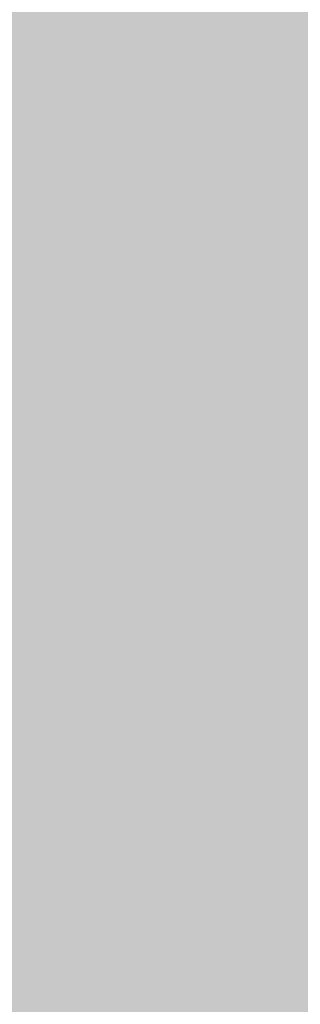
# Model space of a CAD drawing. Units: inches. Extents: x 2083 to 3317, y 1141 to 2115.
# Tile 167 of 256: x 3126.955939 to 3126.958245, y 1263.265937 to 1263.274018. Entities that reach past the tile are written whole.
import ezdxf

# ---------------------------------------------------------------- set-up
doc = ezdxf.new("R2010")
doc.units = ezdxf.units.IN
doc.layers.add('A-ANNO-DIMS', color=2, linetype='Continuous', lineweight=18)
doc.layers.add('A-WALL-PATT', color=251, linetype='Continuous', lineweight=13, true_color=0x636466)
doc.styles.get("Standard").update_dxf_attribs({"font": 'arial.ttf'})
doc.dimstyles.new('ISO-25', dxfattribs={"dimtxt": 12, "dimasz": 12, "dimexe": 1.25, "dimexo": 0.625, "dimtad": 1, "dimlunit": 3, "dimtxsty": 'Standard', "dimcen": 2.5, "dimadec": 0, "dimazin": 0, "dimtfac": 1, "dimtmove": 0, "dimatfit": 3, "dimfxl": 1, "dimarcsym": 0})

# ---------------------------------------------------------------- blocks, each defined once
blk = doc.blocks.new('*D26')
at = {"layer": 'A-ANNO-DIMS', "color": 0, "lineweight": -2, "transparency": 16777216}
for p, q in [((3088.985844, 1274.915092), (3088.985844, 1270.9519631)), ((3111.2400366, 1274.915092), (3111.2400366, 1270.9519631)), ((3076.985844, 1272.2019631), (2840.262447, 1272.2019631)), ((3111.2400366, 1272.2019631), (3088.985844, 1272.2019631)), ((3123.2400366, 1272.2019631), (3135.2400366, 1272.2019631))]:
    blk.add_line(p, q, dxfattribs=at)
at = {"layer": 'A-ANNO-DIMS', "color": 0, "transparency": 16777216}
for points in [[(3076.985844, 1274.2019631), (3076.985844, 1270.2019631), (3088.985844, 1272.2019631)], [(3123.2400366, 1274.2019631), (3123.2400366, 1270.2019631), (3111.2400366, 1272.2019631)]]:
    blk.add_solid(points, dxfattribs=at)
at = {"layer": 'Defpoints', "color": 0, "transparency": 16777216}
for p in [(3088.985844, 1275.540092), (3111.2400366, 1275.540092), (3088.985844, 1272.2019631)]:
    blk.add_point(p, dxfattribs=at)
at = {"layer": 'A-ANNO-DIMS', "color": 0, "transparency": 16777216, "insert": (2952.6241455, 1279.0316016), "char_height": 12, "attachment_point": 5}
blk.add_mtext('NIGHTSTAND 1\'-10 1/2" TYP.', dxfattribs=at)

msp = doc.modelspace()

# ---------------------------------------------------------------- hatches: boundary and pattern name
at = {"layer": 'A-WALL-PATT'}
h = msp.add_hatch(color=256, dxfattribs=at)
h.dxf.hatch_style = 1
h.paths.add_polyline_path([(3126.9597832, 2020.7613601), (2748.9597832, 2020.7613601), (2604.9597832, 2020.7613601), (2226.9597832, 2020.7613601), (2226.9597832, 1702.7613601), (2466.9597832, 1702.7613601), (2466.9597832, 1582.7613601), (2418.9597832, 1582.7613601), (2418.9597832, 1477.7613601), (2226.9597832, 1477.7613601), (2226.9597832, 1263.2613601), (2544.9597832, 1263.2613601), (2544.9597832, 1411.7613601), (2604.9597832, 1411.7613601), (2685.9597832, 1411.7613601), (2685.9597832, 1420.7613601), (2604.9597832, 1420.7613601), (2604.9597832, 1573.7613601), (2604.9597832, 1702.7613601), (2604.9597832, 2011.7613601), (2748.9597832, 2011.7613601), (2748.9597832, 1702.7613601), (2862.9597832, 1702.7613601), (2862.9597832, 1621.7613601), (2871.9597832, 1621.7613601), (2871.9597832, 1702.7613601), (2883.9597832, 1702.7613601), (2883.9597832, 1706.9394595, -0.026459), (2883.9597832, 1711.7613601), (2757.9597832, 1711.7613601), (2757.9597832, 1807.7613601), (2787.9597832, 1807.7613601), (2787.9597832, 1812.2613601), (2757.9597832, 1812.2613601), (2757.9597832, 2011.7613601), (2877.9597832, 2011.7613601), (2877.9597832, 1812.2613601), (2847.9597832, 1812.2613601), (2847.9597832, 1807.7613601), (2889.8357425, 1807.7613601), (2889.8357425, 1812.2613601), (2882.4597832, 1812.2613601), (2882.4597832, 2011.7613601), (3117.9597832, 2011.7613601), (3117.9597832, 1812.2613601), (2937.8357425, 1812.2613601), (2937.8357425, 1807.7613601), (2995.7097832, 1807.7613601), (2995.7097832, 1796.1176655), (3000.2097832, 1796.1176655), (3000.2097832, 1807.7613601), (3117.9597832, 1807.7613601), (3117.9597832, 1711.7613601), (3000.2097832, 1711.7613601), (3000.2097832, 1760.1176655), (2998.5727047, 1760.1176655, -0.020711), (2995.7097832, 1760.1176655), (2995.7097832, 1711.7613601), (2931.9597832, 1711.7613601), (2931.9597832, 1702.7613601), (3126.9597832, 1702.7613601)])
h.paths.add_polyline_path([(2471.4597832, 2011.7613601), (2471.4597832, 1810.0113601), (2462.7169357, 1810.0113601), (2462.7169357, 1805.5113601), (2505.9597832, 1805.5113601), (2505.9597832, 1810.0113601), (2475.9597832, 1810.0113601), (2475.9597832, 2011.7613601), (2595.9597832, 2011.7613601), (2595.9597832, 1810.0113601), (2565.9597832, 1810.0113601), (2565.9597832, 1805.5113601), (2595.9597832, 1805.5113601), (2595.9597832, 1711.7613601), (2235.9597832, 1711.7613601), (2235.9597832, 1805.5113601), (2353.7097832, 1805.5113601), (2353.7097832, 1796.0541624), (2358.2097832, 1796.0541624), (2358.2097832, 1805.5113601), (2414.7169357, 1805.5113601), (2414.7169357, 1810.0113601), (2235.9597832, 1810.0113601), (2235.9597832, 2011.7613601)], flags=16)
h.paths.add_polyline_path([(2270.2047343, 1994.6100082), (2270.2047343, 1970.6100082), (2246.2047343, 1970.6100082), (2246.2047343, 1994.6100082)], flags=0)
edge = h.paths.add_edge_path(flags=0)
edge.add_ellipse((2332.027391, 1899.7981761), major_axis=(-3.0429938, 3.0429938), ratio=0.16825245, start_angle=-161.3321656, end_angle=-156.3071136, ccw=False)
edge.add_ellipse((2333.0820373, 1898.7435297), major_axis=(-1.0546463, 1.0546463), ratio=0.453532097, start_angle=-123.371019, end_angle=-94.1591066)
edge = h.paths.add_edge_path(flags=0)
edge.add_ellipse((2332.027391, 1968.8762897), major_axis=(3.0429938, 3.0429938), ratio=0.16825245, start_angle=18.6678344, end_angle=23.6928864)
edge.add_spline(control_points=[(2332.9255964, 1970.6911045), (2332.2267681, 1970.3360997), (2330.8937087, 1969.6589054), (2328.4130803, 1970.9321376), (2327.2039345, 1967.7487119), (2324.7095965, 1969.9555886), (2322.5328223, 1967.012354), (2320.0128462, 1971.2958124), (2317.6803077, 1968.1578449), (2316.0405263, 1967.1020468), (2315.4269045, 1966.8096022)], knot_values=[0, 0, 0, 0, 2.267059, 4.324559, 6.685584, 8.878641, 11.121502, 14.300359, 17.755284, 19.732645, 19.732645, 19.732645, 19.732645], degree=3, periodic=0)
edge.add_ellipse((2332.027391, 1968.8762897), major_axis=(3.0429938, 3.0429938), ratio=0.16825245, start_angle=18.6678344, end_angle=23.6928864, ccw=False)
edge.add_ellipse((2333.0820373, 1969.930936), major_axis=(1.0546463, 1.0546463), ratio=0.453532097, start_angle=56.628981, end_angle=85.8408934, ccw=False)
edge = h.paths.add_edge_path(flags=0)
edge.add_spline(control_points=[(2296.4282874, 1967.9879081), (2293.6278045, 1965.3363137), (2287.7036238, 1959.727094), (2299.7438601, 1949.9956993), (2294.5325909, 1935.6685275), (2290.5732281, 1920.6035119), (2293.3941244, 1909.9736911), (2296.1854073, 1904.9665431)], knot_values=[0.099185, 0.099185, 0.099185, 0.099185, 0.345301, 0.619822, 0.982653, 1.386093, 1.810555, 1.810555, 1.810555, 1.810555], degree=3, periodic=0)
edge.add_spline(control_points=[(2296.1854073, 1904.9665431), (2297.3835817, 1902.6193002), (2298.0009694, 1901.9493116), (2298.5529698, 1901.4681549)], knot_values=[0.006246, 0.006246, 0.006246, 0.006246, 0.055476, 0.055476, 0.055476, 0.055476], degree=3, periodic=0)
edge.add_spline(control_points=[(2298.5529698, 1901.4681549), (2297.2586121, 1900.9232238), (2295.2252939, 1900.2321257), (2293.0602287, 1900.6142053), (2292.1014227, 1900.788415), (2292.0895776, 1900.790568)], knot_values=[0.312835, 0.312835, 0.312835, 0.312835, 0.40178, 0.474987, 0.475903, 0.475903, 0.475903, 0.475903], degree=3, periodic=0)
edge.add_arc((2292.7936464, 1904.6641088), 3.9370079, 215.4208969, 259.6981795, ccw=False)
edge.add_spline(control_points=[(2289.5853139, 1902.3823039), (2289.4766524, 1902.5350874), (2289.3684805, 1902.6880353), (2289.2608648, 1902.8411699)], knot_values=[0.102872, 0.102872, 0.102872, 0.102872, 0.116896, 0.116896, 0.116896, 0.116896], degree=3, periodic=0)
edge.add_spline(control_points=[(2289.2608648, 1902.8411699), (2288.6866042, 1902.5501922), (2287.6400477, 1902.0199025), (2285.8813368, 1901.8739536), (2283.8529717, 1901.5043521), (2281.7199871, 1899.7105375), (2278.4669913, 1899.492942), (2276.1571361, 1901.8832022), (2272.2589526, 1899.8040711), (2267.7776054, 1901.8431828), (2262.2438819, 1900.1840326), (2257.414927, 1901.7820606), (2254.318374, 1900.7261196), (2253.1782849, 1900.3373431)], knot_values=[0, 0, 0, 0, 1.907977, 3.477176, 5.261074, 7.972851, 11.680248, 13.717921, 16.939592, 22.789562, 27.502503, 33.595215, 37.145618, 37.145618, 37.145618, 37.145618], degree=3, periodic=0)
edge.add_line((2253.1782849, 1900.3373431), (2250.2442397, 1902.8411699))
edge.add_line((2250.2442397, 1902.8411699), (2250.2442397, 1965.8332959))
edge.add_line((2250.2442397, 1965.8332959), (2253.1782849, 1968.3371226))
edge.add_spline(control_points=[(2253.1782849, 1968.3371226), (2254.318374, 1967.9483462), (2257.414927, 1966.8924051), (2262.2438819, 1968.4904332), (2267.7776054, 1966.8312829), (2271.5267301, 1968.5372172), (2273.8759143, 1967.8282895), (2274.2067012, 1967.7276424)], knot_values=[0, 0, 0, 0, 0.09018, 0.244935, 0.364644, 0.513233, 0.537855, 0.537855, 0.537855, 0.537855], degree=3, periodic=0)
edge.add_arc((2274.3528869, 1963.7933495), 3.9370079, 72.0511336, 92.1279492, ccw=False)
edge.add_arc((2281.2969331, 1985.2300027), 18.5962982, 252.05113361, 288.56572166)
edge.add_arc((2292.3167172, 1956.0288805), 12.6460805, 71.02678788, 113.77821843, ccw=False)
edge = h.paths.add_edge_path(flags=0)
edge.add_spline(control_points=[(2274.8994147, 1951.8561946), (2275.066156, 1951.6165924), (2275.2326866, 1951.3765878), (2275.3979871, 1951.1358545)], knot_values=[1.409916, 1.409916, 1.409916, 1.409916, 1.43159, 1.43159, 1.43159, 1.43159], degree=3, periodic=0)
edge.add_spline(control_points=[(2275.3979871, 1951.1358545), (2275.7921055, 1950.5618854), (2276.1792311, 1949.9837745), (2276.5455462, 1949.3971029)], knot_values=[1.358238, 1.358238, 1.358238, 1.358238, 1.409916, 1.409916, 1.409916, 1.409916], degree=3, periodic=0)
edge.add_line((2276.5455462, 1949.3971029), (2277.437289, 1947.8621847))
edge.add_spline(control_points=[(2277.437289, 1947.8621847), (2276.3038341, 1945.6731147), (2274.6396979, 1942.4268817), (2274.631615, 1938.0938998), (2272.7991237, 1930.8515498), (2274.3564261, 1943.8970461), (2275.9476814, 1947.9233558), (2276.5455462, 1949.3971029)], knot_values=[0.005632, 0.005632, 0.005632, 0.005632, 0.186014, 0.266002, 0.357087, 0.59639, 0.739732, 0.739732, 0.739732, 0.739732], degree=3, periodic=0)
edge.add_spline(control_points=[(2276.5455462, 1949.3971029), (2276.1792311, 1949.9837745), (2275.7921055, 1950.5618854), (2275.3979871, 1951.1358545)], knot_values=[1.358238, 1.358238, 1.358238, 1.358238, 1.409916, 1.409916, 1.409916, 1.409916], degree=3, periodic=0)
edge.add_spline(control_points=[(2275.3979871, 1951.1358545), (2274.9425002, 1950.0804523), (2274.2077604, 1948.0252718), (2273.9346018, 1944.8514774), (2272.4685341, 1937.6274891), (2273.4662155, 1945.6964663), (2274.7006154, 1951.0594725), (2274.8994147, 1951.8561946)], knot_values=[0.104364, 0.104364, 0.104364, 0.104364, 0.189636, 0.269624, 0.36071, 0.600013, 0.644622, 0.644622, 0.644622, 0.644622], degree=3, periodic=0)
h.paths.add_polyline_path([(2269.1675139, 1963.1275729, -0.357527), (2268.170633, 1960.9763695, -0.092561), (2268.170633, 1939.4363249, -0.357527), (2269.1675139, 1937.2851215, -0.357527), (2267.0163105, 1938.2820024, -0.164785), (2254.6855813, 1938.2820024, -0.357527), (2252.5343779, 1937.2851215, -0.357527), (2253.5312587, 1939.4363249, -0.092561), (2253.5312587, 1960.9763695, -0.357527), (2252.5343779, 1963.1275729, -0.357527), (2254.6855813, 1962.130692, -0.164785), (2267.0163105, 1962.130692, -0.357527)], flags=0)
h.paths.add_polyline_path([(2248.8740679, 1967.8017998), (2248.8740679, 1957.0277095), (2249.4577833, 1957.0277095), (2249.4577833, 1911.6467562), (2248.8740679, 1911.6467562), (2248.8740679, 1900.8726659), (2246.5118632, 1900.8726659, 0.197327), (2244.1496584, 1902.4568734), (2244.1496584, 1966.2175923, 0.197327), (2246.5118632, 1967.8017998)], flags=0)
h.paths.add_polyline_path([(2269.1675139, 1931.3893442, -0.357527), (2268.170633, 1929.2381408, -0.092561), (2268.170633, 1907.6980962, -0.357527), (2269.1675139, 1905.5468928, -0.357527), (2267.0163105, 1906.5437737, -0.164785), (2254.6855813, 1906.5437737, -0.357527), (2252.5343779, 1905.5468928, -0.357527), (2253.5312587, 1907.6980962, -0.092561), (2253.5312587, 1929.2381408, -0.357527), (2252.5343779, 1931.3893442, -0.357527), (2254.6855813, 1930.3924634, -0.164785), (2267.0163105, 1930.3924634, -0.357527)], flags=0)
edge = h.paths.add_edge_path(flags=0)
edge.add_spline(control_points=[(2276.1968578, 1906.7237016), (2276.1681442, 1909.0289278), (2276.1140492, 1913.371852), (2270.5984171, 1924.9249783), (2273.9051746, 1919.0127787), (2275.9217115, 1916.2620626), (2275.4745699, 1912.4021495), (2277.2578735, 1910.3806206), (2276.6960436, 1908.2250358), (2276.6462176, 1906.8130226), (2276.6178249, 1906.0084068)], knot_values=[0, 0, 0, 0, 8.61026, 16.221274, 18.843057, 23.804898, 27.440828, 29.356102, 31.203478, 33.650687, 33.650687, 33.650687, 33.650687], degree=3, periodic=0)
edge.add_spline(control_points=[(2276.6178249, 1906.0084068), (2276.6233131, 1905.6241436), (2276.4977381, 1904.6286608), (2275.4417789, 1903.8547251), (2274.9373144, 1903.0804497), (2274.8590804, 1902.8411699)], knot_values=[0.156488, 0.156488, 0.156488, 0.156488, 0.184398, 0.231376, 0.250598, 0.250598, 0.250598, 0.250598], degree=3, periodic=0)
edge.add_line((2274.8590804, 1902.8411699), (2276.50598, 1902.8411699))
edge.add_spline(control_points=[(2276.50598, 1902.8411699), (2276.7883084, 1903.0849395), (2277.6650711, 1904.1251958), (2278.2495378, 1904.340738), (2277.6538719, 1908.5273866), (2278.15567, 1906.2278078), (2278.100464, 1905.2859484), (2278.8466748, 1904.0690054), (2277.8567853, 1903.4149482), (2277.8741909, 1902.9910497), (2277.9035616, 1902.8411699)], knot_values=[0.059574, 0.059574, 0.059574, 0.059574, 0.080753, 0.103741, 0.16972, 0.176036, 0.207137, 0.240474, 0.262341, 0.27366, 0.27366, 0.27366, 0.27366], degree=3, periodic=0)
edge.add_line((2277.9035616, 1902.8411699), (2280.0298255, 1902.8411699))
edge.add_spline(control_points=[(2280.0298255, 1902.8411699), (2279.8882214, 1903.088398), (2279.4992571, 1903.9815512), (2280.1522839, 1905.9393491), (2278.103615, 1909.6577572), (2279.7623946, 1907.185285), (2280.3279002, 1904.8748608), (2280.4851086, 1903.4895904), (2281.4632687, 1903.2494323), (2281.7583431, 1902.9364967), (2281.8340361, 1902.8411699)], knot_values=[0.013856, 0.013856, 0.013856, 0.013856, 0.034874, 0.088867, 0.107879, 0.126738, 0.158714, 0.193757, 0.217487, 0.226722, 0.226722, 0.226722, 0.226722], degree=3, periodic=0)
edge.add_spline(control_points=[(2281.8340361, 1902.8411699), (2281.7875348, 1902.8267029), (2281.6470224, 1902.7829881), (2281.3955272, 1902.85949), (2281.088077, 1902.9852418), (2280.7206826, 1903.060902), (2280.3334513, 1903.0257257), (2280.1247668, 1902.898879), (2280.0298255, 1902.8411699)], knot_values=[0, 0, 0, 0, 0.14413, 0.435517, 0.749276, 1.153046, 1.548371, 1.878348, 1.878348, 1.878348, 1.878348], degree=3, periodic=0)
edge.add_line((2280.0298255, 1902.8411699), (2277.9035616, 1902.8411699))
edge.add_spline(control_points=[(2277.9035616, 1902.8411699), (2277.892855, 1902.7958553), (2277.865396, 1902.6796374), (2277.6074793, 1902.6874828), (2277.2740503, 1902.8006999), (2276.8379209, 1902.6197745), (2276.5838074, 1902.7892611), (2276.50598, 1902.8411699)], knot_values=[0, 0, 0, 0, 0.127189, 0.326199, 0.628009, 1.24357, 1.515331, 1.515331, 1.515331, 1.515331], degree=3, periodic=0)
edge.add_line((2276.50598, 1902.8411699), (2274.8590804, 1902.8411699))
edge.add_spline(control_points=[(2274.8590804, 1902.8411699), (2274.8144367, 1902.8985868), (2274.7251297, 1903.013446), (2274.4934765, 1903.1189684), (2274.2442854, 1902.9605386), (2273.9371207, 1903.1849416), (2273.6140395, 1902.9831428), (2273.4083164, 1902.8830449), (2273.322254, 1902.8411699)], knot_values=[0, 0, 0, 0, 0.21843, 0.436957, 0.687977, 0.990379, 1.398396, 1.69185, 1.69185, 1.69185, 1.69185], degree=3, periodic=0)
edge.add_spline(control_points=[(2273.322254, 1902.8411699), (2273.6167403, 1903.445692), (2274.2739977, 1904.5382529), (2276.0272387, 1904.5737017), (2276.2069634, 1906.5836372), (2276.1968578, 1906.7237016)], knot_values=[0.012227, 0.012227, 0.012227, 0.012227, 0.059472, 0.106218, 0.134458, 0.134458, 0.134458, 0.134458], degree=3, periodic=0)
h.paths.add_polyline_path([(2270.7760538, 1897.7898284), (2270.7760538, 1873.7898284), (2246.7760538, 1873.7898284), (2246.7760538, 1897.7898284)], flags=0)
h.paths.add_polyline_path([(2353.7097832, 1760.0050593), (2353.7097832, 1760.0541624), (2358.2097832, 1760.0541624, -0.033729)], flags=0)
h.paths.add_polyline_path([(2321.8191188, 1737.5291862), (2341.9953271, 1737.5291862, -0.414214), (2343.2032727, 1736.3212406), (2343.2032727, 1721.0205964, -0.414214), (2341.9953271, 1719.8126508), (2321.8191188, 1719.8126508, -0.414214), (2320.6111732, 1721.0205964), (2320.6111732, 1736.3212406, -0.414214)], flags=0)
h.paths.add_polyline_path([(2324.2350099, 1736.3212406), (2339.5794359, 1736.3212406, -0.414214), (2341.9953271, 1733.9053494), (2341.9953271, 1725.4497302, -0.414214), (2339.5794359, 1723.033839), (2333.6805885, 1723.033839), (2333.8453172, 1722.0454666, -0.870646), (2335.4253988, 1721.8258934, -0.767327), (2333.922694, 1721.4232449), (2331.2910241, 1721.4232449, -0.767327), (2329.7883193, 1721.8258934, -0.870646), (2331.3684009, 1722.0454666), (2331.5331296, 1723.033839), (2324.2350099, 1723.033839, -0.414214), (2321.8191188, 1725.4497302), (2321.8191188, 1733.9053494, -0.414214)], flags=0)
h.paths.add_polyline_path([(2570.4837892, 1928.6154443), (2589.6837892, 1928.6154443), (2590.1688286, 1928.6154443), (2590.1688286, 1904.9933971), (2570.4837892, 1904.9933971)], flags=0)
h.paths.add_polyline_path([(2574.4473242, 1927.2638215, -1), (2572.8288357, 1927.2638215, -1)], flags=0)
h.paths.add_polyline_path([(2573.0898665, 1926.9408768), (2573.925032, 1927.7760423), (2574.1477428, 1927.5533315), (2573.3125773, 1926.718166)], flags=0)
h.paths.add_polyline_path([(2578.7790648, 1919.7296175, -1), (2571.5916632, 1919.7296175, -1)], flags=0)
h.paths.add_polyline_path([(2578.385364, 1919.7296175, -1), (2571.985364, 1919.7296175, -1)], flags=0)
h.paths.add_polyline_path([(2331.5957638, 1729.4762156, -1), (2333.6179542, 1729.4762156, -1)], flags=0)
h.paths.add_polyline_path([(2578.0342282, 1927.2638215, -1), (2576.4157396, 1927.2638215, -1)], flags=0)
h.paths.add_polyline_path([(2576.6888513, 1927.5310886), (2576.9115621, 1927.7537993), (2577.7467276, 1926.9186339), (2577.5240168, 1926.6959231)], flags=0)
h.paths.add_polyline_path([(2578.1390648, 1909.8595388, -1), (2572.2316632, 1909.8595388, -1)], flags=0)
h.paths.add_polyline_path([(2577.745364, 1909.8595388, -1), (2572.625364, 1909.8595388, -1)], flags=0)
h.paths.add_polyline_path([(2583.7977179, 1927.2638215, -1), (2582.1792294, 1927.2638215, -1)], flags=0)
h.paths.add_polyline_path([(2582.7186487, 1927.7537993), (2583.5538142, 1926.9186339), (2583.3311034, 1926.6959231), (2582.4959379, 1927.5310886)], flags=0)
h.paths.add_polyline_path([(2582.4959379, 1927.5310886), (2582.7186487, 1927.7537993), (2583.5538142, 1926.9186339), (2583.3311034, 1926.6959231)], flags=0)
h.paths.add_polyline_path([(2587.7390648, 1920.5296175, -1), (2581.8316632, 1920.5296175, -1)], flags=0)
h.paths.add_polyline_path([(2587.345364, 1920.5296175, -1), (2582.225364, 1920.5296175, -1)], flags=0)
h.paths.add_polyline_path([(2587.3846219, 1927.2638215, -1), (2585.7661333, 1927.2638215, -1)], flags=0)
h.paths.add_polyline_path([(2586.0819925, 1926.9802469), (2586.917158, 1927.8154124), (2587.1398688, 1927.5927016), (2586.3047033, 1926.7575361)], flags=0)
h.paths.add_polyline_path([(2588.3790648, 1910.6595388, -1), (2581.1916632, 1910.6595388, -1)], flags=0)
h.paths.add_polyline_path([(2587.985364, 1910.6595388, -1), (2581.585364, 1910.6595388, -1)], flags=0)
h.paths.add_polyline_path([(2417.1677288, 1729.4778955), (2437.3439372, 1729.4778955, -0.414214), (2438.5518828, 1728.2699499), (2438.5518828, 1712.9693057, -0.414214), (2437.3439372, 1711.7613601), (2417.1677288, 1711.7613601, -0.414214), (2415.9597832, 1712.9693057), (2415.9597832, 1728.2699499, -0.414214)], flags=0)
h.paths.add_polyline_path([(2419.58362, 1728.2699499), (2434.928046, 1728.2699499, -0.414214), (2437.3439372, 1725.8540587), (2437.3439372, 1717.3984395, -0.414214), (2434.928046, 1714.9825483), (2429.0291985, 1714.9825483), (2429.1939273, 1713.9941758, -0.870646), (2430.7740089, 1713.7746027, -0.767327), (2429.2713041, 1713.3719542), (2426.6396342, 1713.3719542, -0.767327), (2425.1369294, 1713.7746027, -0.870646), (2426.717011, 1713.9941758), (2426.8817397, 1714.9825483), (2419.58362, 1714.9825483, -0.414214), (2417.1677288, 1717.3984395), (2417.1677288, 1725.8540587, -0.414214)], flags=0)
h.paths.add_polyline_path([(2419.58362, 1728.2699499), (2434.928046, 1728.2699499, -0.414214), (2437.3439372, 1725.8540587), (2437.3439372, 1717.3984395, -0.414214), (2434.928046, 1714.9825483), (2429.0291985, 1714.9825483), (2428.3581177, 1719.0090337), (2427.5528206, 1719.0090337), (2426.8817397, 1714.9825483), (2419.58362, 1714.9825483, -0.414214), (2417.1677288, 1717.3984395), (2417.1677288, 1725.8540587, -0.414214)], flags=0)
h.paths.add_polyline_path([(2426.9443739, 1721.4249248, -1), (2428.9665643, 1721.4249248, -1)], flags=0)
h.paths.add_polyline_path([(2475.9597832, 1702.7613601), (2595.9597832, 1702.7613601), (2595.9597832, 1582.7613601), (2475.9597832, 1582.7613601)], flags=16)
h.paths.add_polyline_path([(2427.9597832, 1573.7613601), (2595.9597832, 1573.7613601), (2595.9597832, 1468.7613601), (2595.9597832, 1420.7613601), (2384.4597832, 1420.7613601), (2384.4597832, 1468.7613601), (2427.9597832, 1468.7613601)], flags=16)
h.paths.add_polyline_path([(2379.9597832, 1468.7613601), (2379.9597832, 1420.7613601), (2235.9597832, 1420.7613601), (2235.9597832, 1468.7613601)], flags=16)
h.paths.add_polyline_path([(2317.8159962, 1466.695767), (2337.9922045, 1466.695767, -0.414214), (2339.2001501, 1465.4878214), (2339.2001501, 1450.1871771, -0.414214), (2337.9922045, 1448.9792315), (2317.8159962, 1448.9792315, -0.414214), (2316.6080506, 1450.1871771), (2316.6080506, 1465.4878214, -0.414214)], flags=0)
h.paths.add_polyline_path([(2320.2318874, 1465.4878214), (2335.5763133, 1465.4878214, -0.414214), (2337.9922045, 1463.0719302), (2337.9922045, 1454.616311, -0.414214), (2335.5763133, 1452.2004198), (2329.6774659, 1452.2004198), (2329.8421946, 1451.2120473, -0.870646), (2331.4222762, 1450.9924742, -0.767327), (2329.9195714, 1450.5898257), (2327.2879015, 1450.5898257, -0.767327), (2325.7851967, 1450.9924742, -0.870646), (2327.3652783, 1451.2120473), (2327.530007, 1452.2004198), (2320.2318874, 1452.2004198, -0.414214), (2317.8159962, 1454.616311), (2317.8159962, 1463.0719302, -0.414214)], flags=0)
h.paths.add_polyline_path([(2320.2318874, 1465.4878214), (2335.5763133, 1465.4878214, -0.414214), (2337.9922045, 1463.0719302), (2337.9922045, 1454.616311, -0.414214), (2335.5763133, 1452.2004198), (2329.6774659, 1452.2004198), (2329.006385, 1456.2269051), (2328.2010879, 1456.2269051), (2327.530007, 1452.2004198), (2320.2318874, 1452.2004198, -0.414214), (2317.8159962, 1454.616311), (2317.8159962, 1463.0719302, -0.414214)], flags=0)
h.paths.add_polyline_path([(2327.5926413, 1458.6427963, -1), (2329.6148317, 1458.6427963, -1)], flags=0)
h.paths.add_polyline_path([(2244.4117436, 1433.3404531), (2241.9209449, 1433.3404531, -0.414214), (2240.0178562, 1435.2435418), (2240.0178562, 1440.9528078, -0.414211), (2241.920925, 1442.8558965), (2244.4117436, 1442.8558965, -1.976472)], flags=0)
h.paths.add_polyline_path([(2245.3568884, 1434.3975358, -0.414214), (2245.3568884, 1441.7988138, -2.144098)], flags=0)
h.paths.add_polyline_path([(2535.9597832, 1416.2613601), (2535.9597832, 1272.2613601), (2235.9597832, 1272.2613601), (2235.9597832, 1416.2613601)], flags=16)
h.paths.add_polyline_path([(2260.1195614, 1384.2928413), (2260.1195614, 1362.0386487), (2237.8653688, 1362.0386487), (2237.8653688, 1384.2928413)], flags=0)
edge = h.paths.add_edge_path(flags=0)
edge.add_line((2318.2518466, 1362.0932983), (2318.1457968, 1362.0009726))
edge.add_ellipse((2317.4451158, 1360.4310442), major_axis=(2.8216404, 2.8216404), ratio=0.16825245, start_angle=18.6678344, end_angle=20.9481273, ccw=False)
edge.add_ellipse((2318.4230451, 1361.4089735), major_axis=(0.9779293, 0.9779293), ratio=0.453532097, start_angle=56.628981, end_angle=70.2262012, ccw=False)
edge = h.paths.add_edge_path(flags=0)
edge.add_line((2319.1073699, 1295.5710784), (2319.0150442, 1295.6771282))
edge.add_ellipse((2317.4451158, 1296.3778091), major_axis=(-2.8216404, 2.8216404), ratio=0.16825245, start_angle=-161.3321656, end_angle=-159.0518727, ccw=False)
edge.add_ellipse((2318.4230451, 1295.3998798), major_axis=(-0.9779293, 0.9779293), ratio=0.453532097, start_angle=-123.371019, end_angle=-109.7737988)
edge = h.paths.add_edge_path(flags=0)
edge.add_spline(control_points=[(2284.2103489, 1301.1702189), (2284.5806878, 1300.444719), (2284.8911891, 1299.8920243), (2285.159553, 1299.4610182)], knot_values=[0.039066, 0.039066, 0.039066, 0.039066, 0.055476, 0.055476, 0.055476, 0.055476], degree=3, periodic=0)
edge.add_line((2285.159553, 1299.4610182), (2284.2103489, 1301.1702189))
edge = h.paths.add_edge_path(flags=0)
edge.add_line((2280.4124579, 1297.2980125), (2283.3699905, 1297.0361216))
edge.add_line((2283.3699905, 1297.0361216), (2286.4056902, 1297.9263104))
edge.add_spline(control_points=[(2286.4056902, 1297.9263104), (2285.305487, 1297.4631193), (2284.3447774, 1297.1291508), (2283.3699905, 1297.0361216)], knot_values=[0.394369, 0.394369, 0.394369, 0.394369, 0.475903, 0.475903, 0.475903, 0.475903], degree=3, periodic=0)
edge.add_spline(control_points=[(2283.3699905, 1297.0361216), (2283.2813895, 1297.027666), (2282.316289, 1296.9573356), (2281.3125019, 1297.1344787), (2280.4234414, 1297.2960161), (2280.4124579, 1297.2980125)], knot_values=[0.312835, 0.312835, 0.312835, 0.312835, 0.320246, 0.393453, 0.394369, 0.394369, 0.394369, 0.394369], degree=3, periodic=0)
edge = h.paths.add_edge_path(flags=0)
edge.add_line((2284.4355615, 1359.6072854), (2280.4462909, 1355.328047))
edge.add_line((2280.4462909, 1355.328047), (2279.5799868, 1351.0177544))
edge.add_line((2279.5799868, 1351.0177544), (2282.4129737, 1346.5804327))
edge.add_spline(control_points=[(2282.4129737, 1346.5804327), (2283.1533308, 1345.5892358), (2284.2528957, 1344.0288973), (2284.801037, 1342.3871671), (2284.9351625, 1341.8055443)], knot_values=[1.240098, 1.240098, 1.240098, 1.240098, 1.332892, 1.382712, 1.382712, 1.382712, 1.382712], degree=3, periodic=0)
edge.add_spline(control_points=[(2284.9351625, 1341.8055443), (2285.3191079, 1340.1406002), (2285.2330291, 1338.4092041), (2284.9099384, 1336.6541222)], knot_values=[1.097484, 1.097484, 1.097484, 1.097484, 1.240098, 1.240098, 1.240098, 1.240098], degree=3, periodic=0)
edge.add_spline(control_points=[(2284.9099384, 1336.6541222), (2284.5868478, 1334.8990403), (2284.0267453, 1333.1202725), (2283.4626437, 1331.3605849)], knot_values=[0.95487, 0.95487, 0.95487, 0.95487, 1.097484, 1.097484, 1.097484, 1.097484], degree=3, periodic=0)
edge.add_line((2283.4626437, 1331.3605849), (2281.8903759, 1326.153357))
edge.add_line((2281.8903759, 1326.153357), (2280.7562592, 1321.0560888))
edge.add_line((2280.7562592, 1321.0560888), (2280.2992048, 1316.0019772))
edge.add_line((2280.2992048, 1316.0019772), (2280.7159327, 1310.9500678))
edge.add_line((2280.7159327, 1310.9500678), (2282.0280939, 1305.9721367))
edge.add_line((2282.0280939, 1305.9721367), (2284.2103489, 1301.1702189))
edge.add_spline(control_points=[(2284.2103489, 1301.1702189), (2283.3407305, 1302.7301854), (2282.6119044, 1304.3364933), (2282.0280939, 1305.9721367)], knot_values=[0.099185, 0.099185, 0.099185, 0.099185, 0.241799, 0.241799, 0.241799, 0.241799], degree=3, periodic=0)
edge.add_spline(control_points=[(2282.0280939, 1305.9721367), (2281.4442835, 1307.6077801), (2281.0054886, 1309.2727591), (2280.7159327, 1310.9500678)], knot_values=[0.241799, 0.241799, 0.241799, 0.241799, 0.384413, 0.384413, 0.384413, 0.384413], degree=3, periodic=0)
edge.add_spline(control_points=[(2280.7159327, 1310.9500678), (2280.4332411, 1312.5876134), (2280.2893863, 1314.2769594), (2280.2988938, 1315.9620324), (2280.2992048, 1316.0019772)], knot_values=[0.384413, 0.384413, 0.384413, 0.384413, 0.523647, 0.527028, 0.527028, 0.527028, 0.527028], degree=3, periodic=0)
edge.add_spline(control_points=[(2280.2992048, 1316.0019772), (2280.3123257, 1317.6869552), (2280.4778706, 1319.3679256), (2280.7562592, 1321.0560888)], knot_values=[0.527028, 0.527028, 0.527028, 0.527028, 0.669642, 0.669642, 0.669642, 0.669642], degree=3, periodic=0)
edge.add_spline(control_points=[(2280.7562592, 1321.0560888), (2281.0346478, 1322.7442519), (2281.4258801, 1324.4396079), (2281.8903759, 1326.153357)], knot_values=[0.669642, 0.669642, 0.669642, 0.669642, 0.812256, 0.812256, 0.812256, 0.812256], degree=3, periodic=0)
edge.add_spline(control_points=[(2281.8903759, 1326.153357), (2282.2643834, 1327.5332507), (2282.7878702, 1329.2618097), (2283.352751, 1331.0177803), (2283.4626437, 1331.3605849)], knot_values=[0.812256, 0.812256, 0.812256, 0.812256, 0.927087, 0.95487, 0.95487, 0.95487, 0.95487], degree=3, periodic=0)
edge.add_line((2283.4626437, 1331.3605849), (2284.9099384, 1336.6541222))
edge.add_line((2284.9099384, 1336.6541222), (2284.9351625, 1341.8055443))
edge.add_line((2284.9351625, 1341.8055443), (2282.4129737, 1346.5804327))
edge.add_spline(control_points=[(2282.4129737, 1346.5804327), (2281.2751273, 1348.1037918), (2280.0784467, 1349.5703178), (2279.5799868, 1351.0177544)], knot_values=[1.382712, 1.382712, 1.382712, 1.382712, 1.525326, 1.525326, 1.525326, 1.525326], degree=3, periodic=0)
edge.add_spline(control_points=[(2279.5799868, 1351.0177544), (2279.4432818, 1351.4147209), (2279.1363124, 1352.856922), (2279.7351897, 1354.2903851), (2280.4462909, 1355.328047)], knot_values=[1.525326, 1.525326, 1.525326, 1.525326, 1.564439, 1.667941, 1.667941, 1.667941, 1.667941], degree=3, periodic=0)
edge.add_spline(control_points=[(2280.4462909, 1355.328047), (2281.4261132, 1356.7578354), (2282.9308373, 1358.1825604), (2284.4355615, 1359.6072854)], knot_values=[1.667941, 1.667941, 1.667941, 1.667941, 1.810555, 1.810555, 1.810555, 1.810555], degree=3, periodic=0)
edge.add_arc((2280.6230749, 1348.518181), 11.7261796, 71.02678788, 113.77821843)
edge.add_arc((2270.4048917, 1375.5951559), 17.2435667, 252.05113361, 288.56572166, ccw=False)
edge.add_arc((2263.9659692, 1355.7178471), 3.6506221, 72.0511336, 92.1279492)
edge.add_arc((2263.9659692, 1355.7178471), 3.6506221, 92.1279492, 177.98513)
edge.add_spline(control_points=[(2260.3176041, 1355.8461989), (2260.2604169, 1354.2206683), (2260.551278, 1350.1865469), (2262.9993445, 1346.7662507), (2264.4727415, 1344.6490245)], knot_values=[1.43159, 1.43159, 1.43159, 1.43159, 1.564144, 1.770695, 1.770695, 1.770695, 1.770695], degree=3, periodic=0)
edge.add_line((2264.4727415, 1344.6490245), (2264.9355904, 1343.9825301))
edge.add_spline(control_points=[(2263.8010444, 1340.2481052), (2263.8432379, 1340.5140884), (2264.0672444, 1341.7564652), (2264.5126928, 1343.0024532), (2264.9350468, 1343.9810834)], knot_values=[0.53657, 0.53657, 0.53657, 0.53657, 0.559349, 0.644622, 0.644622, 0.644622, 0.644622], degree=3, periodic=0)
edge.add_spline(control_points=[(2264.9350468, 1343.9810834), (2265.1177715, 1343.7149747), (2265.2988751, 1343.4479058), (2265.4767562, 1343.1793646)], knot_values=[1.384077, 1.384077, 1.384077, 1.384077, 1.409916, 1.409916, 1.409916, 1.409916], degree=3, periodic=0)
edge.add_spline(control_points=[(2265.4767562, 1343.1793646), (2265.6546373, 1342.9108234), (2265.8292958, 1342.64081), (2265.9991301, 1342.368812)], knot_values=[1.358238, 1.358238, 1.358238, 1.358238, 1.384077, 1.384077, 1.384077, 1.384077], degree=3, periodic=0)
edge.add_line((2265.9991301, 1342.368812), (2266.8260057, 1340.9455468))
edge.add_spline(control_points=[(2266.8260057, 1340.9455468), (2268.894401, 1337.0896912), (2271.3981727, 1325.8430009), (2270.5161644, 1310.5685568), (2275.9193759, 1301.860609), (2277.7895113, 1299.1994495)], knot_values=[0.116896, 0.116896, 0.116896, 0.116896, 0.472987, 1.050969, 1.313793, 1.313793, 1.313793, 1.313793], degree=3, periodic=0)
edge.add_spline(control_points=[(2277.7895113, 1299.1994495), (2277.8394051, 1299.1284519), (2277.8894277, 1299.0574975), (2277.9395717, 1298.9865839)], knot_values=[0.109884, 0.109884, 0.109884, 0.109884, 0.116896, 0.116896, 0.116896, 0.116896], degree=3, periodic=0)
edge.add_line((2277.9395717, 1298.9865839), (2277.7888489, 1299.1991139))
edge.add_spline(control_points=[(2277.7888489, 1299.1991139), (2277.2565819, 1298.9294144), (2276.2863504, 1298.4379024), (2275.0393517, 1298.3344186), (2274.3833299, 1298.2388951), (2274.2152543, 1298.209338)], knot_values=[33.12187, 33.12187, 33.12187, 33.12187, 35.029056, 36.598255, 37.144827, 37.144827, 37.144827, 37.144827], degree=3, periodic=0)
edge.add_line((2274.2152543, 1298.209338), (2273.073147, 1297.8929607))
edge.add_spline(control_points=[(2273.073147, 1297.8929607), (2272.3229363, 1297.579784), (2271.0391507, 1296.5105078), (2269.2483948, 1296.2260622), (2268.4231004, 1296.3746543)], knot_values=[26.532584, 26.532584, 26.532584, 26.532584, 29.198919, 31.839101, 31.839101, 31.839101, 31.839101], degree=3, periodic=0)
edge.add_line((2268.4231004, 1296.3746543), (2263.8785014, 1297.4575338))
edge.add_spline(control_points=[(2263.8785014, 1297.4575338), (2263.5560769, 1297.3594345), (2261.8603064, 1296.8386943), (2260.2387805, 1297.2824073), (2258.9334543, 1297.5164611)], knot_values=[15.919551, 15.919551, 15.919551, 15.919551, 16.939592, 21.226067, 21.226067, 21.226067, 21.226067], degree=3, periodic=0)
edge.add_line((2258.9334543, 1297.5164611), (2254.0552332, 1297.3290098))
edge.add_spline(control_points=[(2254.0552332, 1297.3290098), (2253.7555255, 1297.295815), (2252.1136834, 1297.1651738), (2250.4618687, 1297.5442209), (2249.1296862, 1297.6678818)], knot_values=[5.306517, 5.306517, 5.306517, 5.306517, 6.276435, 10.613034, 10.613034, 10.613034, 10.613034], degree=3, periodic=0)
edge.add_line((2249.1296862, 1297.6678818), (2244.3316495, 1296.8777561))
edge.add_line((2244.3316495, 1296.8777561), (2241.6110326, 1299.1994495))
edge.add_line((2241.6110326, 1299.1994495), (2241.6110326, 1357.6094038))
edge.add_line((2241.6110326, 1357.6094038), (2244.3316495, 1359.9310973))
edge.add_line((2244.3316495, 1359.9310973), (2252.7288228, 1359.5426917))
edge.add_spline(control_points=[(2252.7288228, 1359.5426917), (2252.8709387, 1359.5464396), (2253.3057402, 1359.5481716), (2253.7398447, 1359.5142744), (2254.0317419, 1359.4824261)], knot_values=[0.233291, 0.233291, 0.233291, 0.233291, 0.244935, 0.268927, 0.268927, 0.268927, 0.268927], degree=3, periodic=0)
edge.add_line((2254.0317419, 1359.4824261), (2259.5871899, 1359.4163899))
edge.add_spline(control_points=[(2259.5871899, 1359.4163899), (2260.6770676, 1359.6285026), (2262.0731971, 1359.8970025), (2263.5236925, 1359.4592776), (2263.8304173, 1359.3659518)], knot_values=[0.422516, 0.422516, 0.422516, 0.422516, 0.513233, 0.537855, 0.537855, 0.537855, 0.537855], degree=3, periodic=0)
edge.add_arc((2263.9659692, 1355.7178471), 3.6506221, 72.0511336, 92.1279492, ccw=False)
edge.add_arc((2270.4048917, 1375.5951559), 17.2435667, 252.05113361, 288.56572166)
edge.add_arc((2280.6230749, 1348.518181), 11.7261796, 71.02678788, 113.77821843, ccw=False)
h.paths.add_polyline_path([(2240.3405298, 1359.4347149), (2240.3405298, 1349.4443532), (2240.8817846, 1349.4443532), (2240.8817846, 1307.3645001), (2240.3405298, 1307.3645001), (2240.3405298, 1297.3741385), (2238.1501565, 1297.3741385, 0.197327), (2235.9597832, 1298.8431076), (2235.9597832, 1357.9657458, 0.197327), (2238.1501565, 1359.4347149)], flags=0)
h.paths.add_polyline_path([(2259.1577904, 1355.1005005, -0.357527), (2258.2334246, 1353.1057799, -0.092561), (2258.2334246, 1333.1326007, -0.357527), (2259.1577904, 1331.1378801, -0.357527), (2257.1630698, 1332.0622458, -0.164785), (2245.7293022, 1332.0622458, -0.357527), (2243.7345816, 1331.1378801, -0.357527), (2244.6589474, 1333.1326007, -0.092561), (2244.6589474, 1353.1057799, -0.357527), (2243.7345816, 1355.1005005, -0.357527), (2245.7293022, 1354.1761347, -0.164785), (2257.1630698, 1354.1761347, -0.357527)], flags=0)
edge = h.paths.add_edge_path(flags=0)
edge.add_line((2265.9991301, 1342.368812), (2266.8260057, 1340.9455468))
edge.add_line((2266.8260057, 1340.9455468), (2265.3075567, 1337.8140664))
edge.add_line((2265.3075567, 1337.8140664), (2264.358232, 1334.6529388))
edge.add_line((2264.358232, 1334.6529388), (2264.2620123, 1333.7997046))
edge.add_spline(control_points=[(2264.2620123, 1333.7997046), (2264.2083565, 1333.187055), (2264.1620602, 1332.3655252), (2264.0071444, 1331.4139326), (2263.9690487, 1331.2018338)], knot_values=[0.464444, 0.464444, 0.464444, 0.464444, 0.516691, 0.531608, 0.531608, 0.531608, 0.531608], degree=3, periodic=0)
edge.add_spline(control_points=[(2263.9690487, 1331.2018338), (2263.7745349, 1330.1188727), (2263.4243703, 1328.7908386), (2263.2574202, 1328.5306516), (2263.2340282, 1328.5146115)], knot_values=[0.372682, 0.372682, 0.372682, 0.372682, 0.44885, 0.464444, 0.464444, 0.464444, 0.464444], degree=3, periodic=0)
edge.add_spline(control_points=[(2263.2340282, 1328.5146115), (2263.096382, 1328.4202271), (2263.1311696, 1329.3014765), (2263.2749528, 1330.6157493)], knot_values=[0.280919, 0.280919, 0.280919, 0.280919, 0.372682, 0.372682, 0.372682, 0.372682], degree=3, periodic=0)
edge.add_spline(control_points=[(2263.2749528, 1330.6157493), (2263.4187361, 1331.930022), (2263.6715151, 1333.677318), (2263.9698519, 1335.3150268)], knot_values=[0.189157, 0.189157, 0.189157, 0.189157, 0.280919, 0.280919, 0.280919, 0.280919], degree=3, periodic=0)
edge.add_spline(control_points=[(2263.9698519, 1335.3150268), (2264.1004958, 1336.0321917), (2264.4187827, 1337.6219113), (2264.7548476, 1338.8644304), (2264.9474193, 1339.4911244)], knot_values=[0.097394, 0.097394, 0.097394, 0.097394, 0.137578, 0.189157, 0.189157, 0.189157, 0.189157], degree=3, periodic=0)
edge.add_spline(control_points=[(2264.9474193, 1339.4911244), (2265.2900171, 1340.6060546), (2265.6442376, 1341.4939958), (2265.9991301, 1342.368812)], knot_values=[0.005632, 0.005632, 0.005632, 0.005632, 0.097394, 0.097394, 0.097394, 0.097394], degree=3, periodic=0)
h.paths.add_polyline_path([(2259.1577904, 1325.6709733, -0.357527), (2258.2334246, 1323.6762527, -0.092561), (2258.2334246, 1303.7030735, -0.357527), (2259.1577904, 1301.7083529, -0.357527), (2257.1630698, 1302.6327186, -0.164785), (2245.7293022, 1302.6327186, -0.357527), (2243.7345816, 1301.7083529, -0.357527), (2244.6589474, 1303.7030735, -0.092561), (2244.6589474, 1323.6762527, -0.357527), (2243.7345816, 1325.6709733, -0.357527), (2245.7293022, 1324.7466075, -0.164785), (2257.1630698, 1324.7466075, -0.357527)], flags=0)
edge = h.paths.add_edge_path(flags=0)
edge.add_spline(control_points=[(2261.7089377, 1317.3114208), (2261.6794818, 1317.4175798), (2261.7618581, 1317.3885347), (2262.4907358, 1316.0898725), (2262.962185, 1315.3008975)], knot_values=[14.955861, 14.955861, 14.955861, 14.955861, 16.221274, 18.694826, 18.694826, 18.694826, 18.694826], degree=3, periodic=0)
edge.add_spline(control_points=[(2262.962185, 1315.3008975), (2262.9904374, 1315.2536169), (2263.7020958, 1314.0673762), (2264.3489834, 1313.1271533), (2264.7300545, 1312.1641544)], knot_values=[18.694826, 18.694826, 18.694826, 18.694826, 18.843057, 22.433791, 22.433791, 22.433791, 22.433791], degree=3, periodic=0)
edge.add_spline(control_points=[(2264.7300545, 1312.1641544), (2264.8755649, 1311.7964373), (2265.1768733, 1310.7698073), (2265.1430689, 1309.5592623), (2265.2477363, 1308.8241926)], knot_values=[22.433791, 22.433791, 22.433791, 22.433791, 23.804898, 26.172756, 26.172756, 26.172756, 26.172756], degree=3, periodic=0)
edge.add_line((2265.2477363, 1308.8241926), (2265.8507741, 1307.1718879))
edge.add_spline(control_points=[(2265.8507741, 1307.1718879), (2266.0650246, 1306.8216779), (2266.3843872, 1306.3322461), (2266.4244001, 1305.7805489), (2266.4203688, 1305.6112163)], knot_values=[28.062562, 28.062562, 28.062562, 28.062562, 29.356102, 29.911721, 29.911721, 29.911721, 29.911721], degree=3, periodic=0)
edge.add_spline(control_points=[(2266.4203688, 1305.6112163), (2266.4161162, 1305.4325896), (2266.393999, 1305.2499979), (2266.3647773, 1305.0658571)], knot_values=[29.911721, 29.911721, 29.911721, 29.911721, 30.497837, 30.497837, 30.497837, 30.497837], degree=3, periodic=0)
edge.add_line((2266.3647773, 1305.0658571), (2266.0661511, 1302.1362954))
edge.add_spline(control_points=[(2266.0661511, 1302.1362954), (2266.0712401, 1301.7799843), (2265.9980761, 1301.1999847), (2265.6632664, 1300.7589613), (2265.5089084, 1300.5858824)], knot_values=[0.156488, 0.156488, 0.156488, 0.156488, 0.184398, 0.203543, 0.203543, 0.203543, 0.203543], degree=3, periodic=0)
edge.add_line((2265.5089084, 1300.5858824), (2264.4353411, 1299.1994495))
edge.add_line((2264.4353411, 1299.1994495), (2265.962442, 1299.1994495))
edge.add_line((2265.962442, 1299.1994495), (2267.3359898, 1301.1752758))
edge.add_line((2267.3359898, 1301.1752758), (2267.3116668, 1301.9862366))
edge.add_spline(control_points=[(2267.3116668, 1301.9862366), (2267.261111, 1302.8623959), (2267.1602121, 1303.7371316), (2267.2714865, 1303.3258962)], knot_values=[0.126229, 0.126229, 0.126229, 0.126229, 0.166617, 0.166617, 0.166617, 0.166617], degree=3, periodic=0)
edge.add_spline(control_points=[(2267.2714865, 1303.3258962), (2267.2800347, 1303.2943047), (2267.3097851, 1303.1753659), (2267.3734504, 1302.8836084), (2267.4061233, 1302.6828291), (2267.4179259, 1302.6010251)], knot_values=[0.166617, 0.166617, 0.166617, 0.166617, 0.16972, 0.176036, 0.180765, 0.180765, 0.180765, 0.180765], degree=3, periodic=0)
edge.add_spline(control_points=[(2267.7438914, 1300.9875045), (2267.6875832, 1301.1509426), (2267.4805198, 1301.6566644), (2267.4837514, 1302.1447877), (2267.4179259, 1302.6010251)], knot_values=[0.180765, 0.180765, 0.180765, 0.180765, 0.193767, 0.220139, 0.220139, 0.220139, 0.220139], degree=3, periodic=0)
edge.add_line((2267.4179259, 1302.6010251), (2267.7438914, 1300.9875045))
edge.add_spline(control_points=[(2267.7438914, 1300.9875045), (2267.8319608, 1300.7318778), (2267.9320205, 1300.3099042), (2267.5548409, 1299.9745185), (2267.429366, 1299.8292073)], knot_values=[0.220139, 0.220139, 0.220139, 0.220139, 0.240474, 0.25489, 0.25489, 0.25489, 0.25489], degree=3, periodic=0)
edge.add_line((2267.429366, 1299.8292073), (2267.2583608, 1299.1994495))
edge.add_line((2267.2583608, 1299.1994495), (2269.229956, 1299.1994495))
edge.add_spline(control_points=[(2269.229956, 1299.1994495), (2269.0986525, 1299.4286938), (2268.842774, 1300.0162509), (2269.0115749, 1300.9159235), (2268.9467957, 1301.6607397)], knot_values=[0.013856, 0.013856, 0.013856, 0.013856, 0.034874, 0.067073, 0.067073, 0.067073, 0.067073], degree=3, periodic=0)
edge.add_line((2268.9467957, 1301.6607397), (2268.4315815, 1303.6031089))
edge.add_spline(control_points=[(2268.4315815, 1303.6031089), (2268.1755957, 1304.1923747), (2267.5962136, 1305.2512977), (2268.0406981, 1304.6232098), (2268.2513938, 1304.2824205)], knot_values=[0.090155, 0.090155, 0.090155, 0.090155, 0.107879, 0.120289, 0.120289, 0.120289, 0.120289], degree=3, periodic=0)
edge.add_spline(control_points=[(2268.2513938, 1304.2824205), (2268.3608818, 1304.1053294), (2269.0577527, 1302.9179833), (2269.382691, 1301.5904186), (2269.5214051, 1300.7759312), (2269.5752202, 1300.5557836)], knot_values=[0.120289, 0.120289, 0.120289, 0.120289, 0.126738, 0.158714, 0.173506, 0.173506, 0.173506, 0.173506], degree=3, periodic=0)
edge.add_line((2269.5752202, 1300.5557836), (2270.6857984, 1299.4212579))
edge.add_spline(control_points=[(2270.6857984, 1299.4212579), (2270.7672206, 1299.3572512), (2270.8378523, 1299.2814011), (2270.9029248, 1299.1994495)], knot_values=[0.21816, 0.21816, 0.21816, 0.21816, 0.226722, 0.226722, 0.226722, 0.226722], degree=3, periodic=0)
edge.add_line((2270.9372012, 1299.1929131), (2270.9029248, 1299.1994495))
edge.add_spline(control_points=[(2270.9029248, 1299.1994495), (2270.8598061, 1299.1860349), (2270.7295148, 1299.1455), (2270.4963139, 1299.216437), (2270.2716612, 1299.3083234), (2270.1210168, 1299.3479612), (2270.0633386, 1299.3595566)], knot_values=[0.939174, 0.939174, 0.939174, 0.939174, 1.083304, 1.374691, 1.68845, 1.878348, 1.878348, 1.878348, 1.878348], degree=3, periodic=0)
edge.add_line((2270.0633386, 1299.3595566), (2269.229956, 1299.1994495))
edge.add_line((2269.229956, 1299.1994495), (2267.2583608, 1299.1994495))
edge.add_spline(control_points=[(2267.2583608, 1299.1994495), (2267.248433, 1299.1574312), (2267.2229714, 1299.0496673), (2266.9838161, 1299.056942), (2266.8092097, 1299.1162303), (2266.6769047, 1299.1090913), (2266.636531, 1299.1048147)], knot_values=[0.757665, 0.757665, 0.757665, 0.757665, 0.884854, 1.083864, 1.385675, 1.515331, 1.515331, 1.515331, 1.515331], degree=3, periodic=0)
edge.add_spline(control_points=[(2266.636531, 1299.1048147), (2266.4852248, 1299.0887878), (2266.2358066, 1299.0171229), (2266.0346081, 1299.1513168), (2265.962442, 1299.1994495)], knot_values=[0, 0, 0, 0, 0.485905, 0.757665, 0.757665, 0.757665, 0.757665], degree=3, periodic=0)
edge.add_line((2265.962442, 1299.1994495), (2264.4353411, 1299.1994495))
edge.add_line((2264.4353411, 1299.1994495), (2263.8584442, 1299.3671176))
edge.add_spline(control_points=[(2263.8584442, 1299.3671176), (2263.8189433, 1299.3709053), (2263.7795277, 1299.3857212), (2263.7401308, 1299.4015039)], knot_values=[0.845925, 0.845925, 0.845925, 0.845925, 0.978627, 0.978627, 0.978627, 0.978627], degree=3, periodic=0)
edge.add_line((2263.7217862, 1299.3964251), (2263.0103065, 1299.1994495))
edge.add_spline(control_points=[(2263.0103065, 1299.1994495), (2263.2457942, 1299.682859), (2263.5060317, 1300.1281072), (2263.8734943, 1300.4080279)], knot_values=[0.012227, 0.012227, 0.012227, 0.012227, 0.052971, 0.052971, 0.052971, 0.052971], degree=3, periodic=0)
edge.add_spline(control_points=[(2263.8734943, 1300.4080279), (2263.932131, 1300.4526954), (2264.0842429, 1300.5529789), (2264.2551889, 1300.6242227), (2264.3596855, 1300.6647475)], knot_values=[0.052971, 0.052971, 0.052971, 0.052971, 0.059472, 0.069086, 0.069086, 0.069086, 0.069086], degree=3, periodic=0)
edge.add_line((2264.3596855, 1300.6647475), (2265.1418998, 1301.0777737))
edge.add_line((2265.1418998, 1301.0777737), (2265.675806, 1302.7995583))
edge.add_line((2265.675806, 1302.7995583), (2265.5407004, 1305.7040662))
edge.add_line((2265.5407004, 1305.7040662), (2264.8030733, 1309.3277237))
edge.add_line((2264.8030733, 1309.3277237), (2263.0405349, 1314.0917906))
edge.add_spline(control_points=[(2263.0405349, 1314.0917906), (2262.3835724, 1315.6714379), (2261.7959724, 1316.9977489), (2261.7089377, 1317.3114208)], knot_values=[11.216896, 11.216896, 11.216896, 11.216896, 14.955861, 14.955861, 14.955861, 14.955861], degree=3, periodic=0)
h.paths.add_polyline_path([(2871.9597832, 1416.2613601), (2895.910047, 1416.2613601), (2895.910047, 1420.7613601), (2871.9597832, 1420.7613601), (2871.9597832, 1501.7613601), (2862.9597832, 1501.7613601), (2862.9597832, 1420.7613601), (2805.9597832, 1420.7613601), (2805.9597832, 1411.7613601), (2862.9597832, 1411.7613601), (2862.9597832, 1263.2613601), (3126.9597832, 1263.2613601), (3126.9597832, 1411.7613601), (3126.9597832, 1486.7613601), (2943.9597832, 1486.7613601), (2943.9597832, 1477.7613601), (2967.8603109, 1477.7613601), (2967.8603109, 1420.7613601), (2943.910047, 1420.7613601), (2943.910047, 1416.2613601), (3117.9597832, 1416.2613601), (3117.9597832, 1420.7613601), (2972.3603109, 1420.7613601), (2972.3603109, 1477.7613601), (3117.9597832, 1477.7613601), (3117.9597832, 1420.7613601), (3117.9597832, 1272.2613601), (2871.9597832, 1272.2613601)], flags=0)
h.paths.add_polyline_path([(2457.1256256, 1485.9425054), (2527.6026508, 1485.9425054), (2527.6026508, 1537.6357021), (2457.1256256, 1537.6357021)], flags=8)
h.paths.add_polyline_path([(2481.0050583, 1609.9818039), (2590.765818, 1609.9818039), (2590.765818, 1682.0033623), (2481.0050583, 1682.0033623)], flags=8)
h.paths.add_polyline_path([(2483.0850224, 1729.1267835), (2553.5620476, 1729.1267835), (2553.5620476, 1780.8199802), (2483.0850224, 1780.8199802)], flags=8)
h = msp.add_hatch(color=256, dxfattribs=at)
h.dxf.hatch_style = 1
h.paths.add_polyline_path([(3126.9597832, 1486.7613601), (2943.9597832, 1486.7613601), (2943.9597832, 1477.7613601), (2967.8603109, 1477.7613601), (2967.8603109, 1420.7613601), (2943.910047, 1420.7613601), (2943.910047, 1416.2613601), (3117.9597832, 1416.2613601), (3117.9597832, 1420.7613601), (2972.3603109, 1420.7613601), (2972.3603109, 1477.7613601), (3117.9597832, 1477.7613601), (3117.9597832, 1420.7613601), (3117.9597832, 1272.2613601), (2871.9597832, 1272.2613601), (2871.9597832, 1416.2613601), (2895.910047, 1416.2613601), (2895.910047, 1420.7613601), (2871.9597832, 1420.7613601), (2871.9597832, 1501.7613601), (2862.9597832, 1501.7613601), (2862.9597832, 1420.7613601), (2805.9597832, 1420.7613601), (2805.9597832, 1411.7613601), (2862.9597832, 1411.7613601), (2862.9597832, 1263.2613601), (3126.9597832, 1263.2613601), (3126.9597832, 1411.7613601)])

# ---------------------------------------------------------------- dimensions: what is measured, and where the dimension line sits
at = {"layer": 'A-ANNO-DIMS'}
dim = msp.add_linear_dim(base=(3088.985844, 1272.2019631), p1=(3111.2400366, 1275.540092), p2=(3088.985844, 1275.540092), angle=180, text='NIGHTSTAND <> TYP.', dimstyle='ISO-25', override={"dimdec": 1, "dimlfac": 1, "dimrnd": 0, "dimzin": 1, "dimdsep": 46, "dimlunit": 4, "dimfrac": 2}, dxfattribs=at)
dim.commit()
dim.dimension.update_dxf_attribs({"geometry": '*D26', "text_midpoint": (2952.6241455, 1279.0316016)})

doc.saveas('drawing.dxf')
